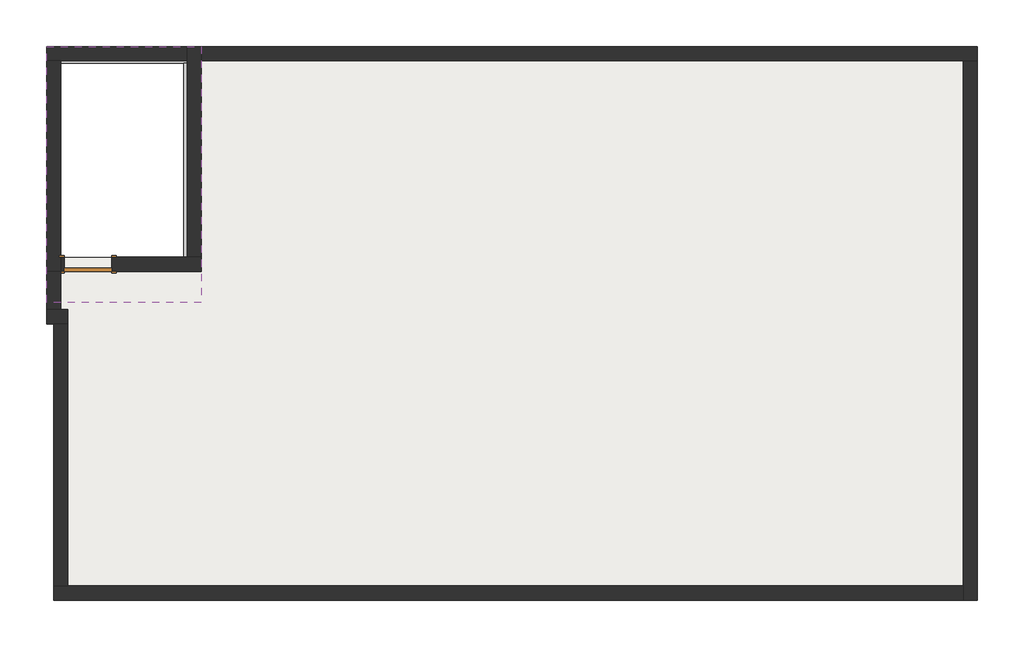
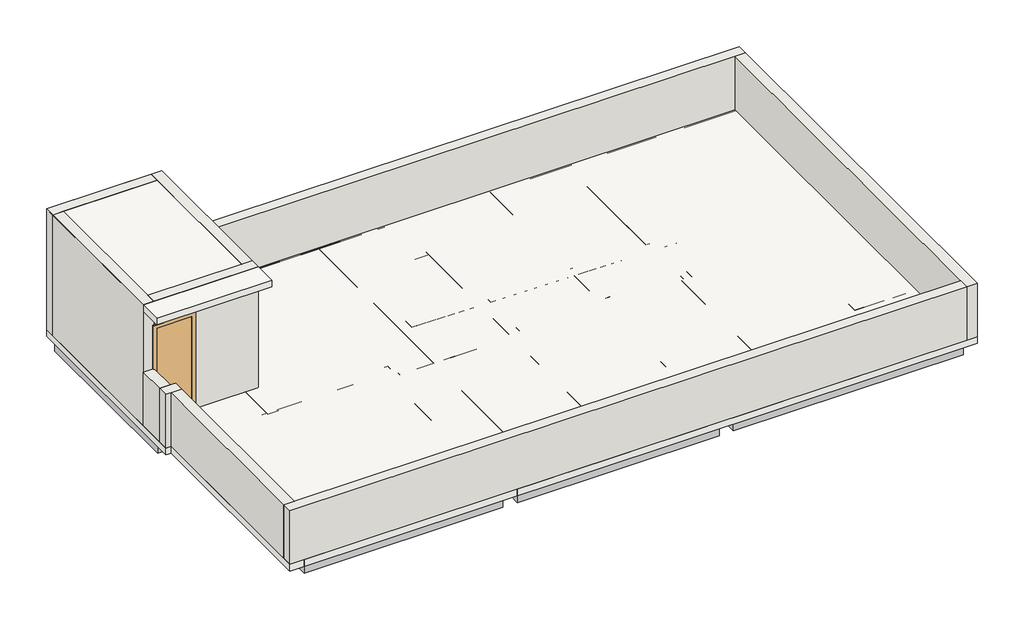
# One storey: 16 beams, 10 walls, 2 slabs, 1 door.
"""IFC4 building model written with IfcOpenShell, lengths in millimetres."""

from ifc_helpers import new_model, si_unit, frame, origin, place, context, project, spatial, polyline, outline, extrude, faceted_brep, transform, mapped, element, save
from components import door_bb98abfd

model = new_model("IFC4")

# Units and contexts
model_context = context("Model", 3, world=origin())
ifc_project = project(units=[si_unit("LENGTHUNIT", "METRE", prefix="MILLI")], contexts=[model_context])

# Site, building, storey
site = spatial("IfcSite", under=ifc_project)
building = spatial("IfcBuilding", under=site)
storey = spatial("IfcBuildingStorey", under=building, Elevation=10210.8)

# Beams
placement = place(None, origin())
element("IfcBeam", 1, ObjectType="Concrete-Rectangular Beam", at=placement, inside=storey, context=model_context, shape_type="Brep", body=[
    faceted_brep([(-12643.368339, 9510.993496, 10210.8), (-12643.368339, 9282.393496, 10210.8), (-10681.218339, 9282.393496, 10210.8), (-10452.618339, 9282.393496, 10210.8), (-7176.018339, 9282.393496, 10210.8), (-6947.418339, 9282.393496, 10210.8), (-5499.618339, 9282.393496, 10210.8), (-5271.018339, 9282.393496, 10210.8), (-3492.916739, 9282.393496, 10210.8), (-3264.316739, 9282.393496, 10210.8), (-1842.018339, 9282.393496, 10210.8), (-1613.418339, 9282.393496, 10210.8), (1790.181661, 9282.393496, 10210.8), (1790.181661, 9510.993496, 10210.8), (-1575.318339, 9510.993496, 10210.8), (-1575.318339, 9320.493496, 10210.8), (-1880.118339, 9320.493496, 10210.8), (-1880.118339, 9510.993496, 10210.8), (-6909.318339, 9510.993496, 10210.8), (-6909.318339, 9320.493496, 10210.8), (-7214.118339, 9320.493496, 10210.8), (-7214.118339, 9510.993496, 10210.8), (-10414.518339, 9510.993496, 10210.8), (-10414.518339, 9320.493496, 10210.8), (-10719.318339, 9320.493496, 10210.8), (-10719.318339, 9510.993496, 10210.8), (-12643.368339, 9282.393496, 9906.0), (-10681.218339, 9282.393496, 9906.0), (-10452.618339, 9282.393496, 9906.0), (-7176.018339, 9282.393496, 9906.0), (-6947.418339, 9282.393496, 9906.0), (-5499.618339, 9282.393496, 9906.0), (-5271.018339, 9282.393496, 9906.0), (-3492.916739, 9282.393496, 9906.0), (-3264.316739, 9282.393496, 9906.0), (-1842.018339, 9282.393496, 9906.0), (-1613.418339, 9282.393496, 9906.0), (1790.181661, 9282.393496, 9906.0), (-12643.368339, 9510.993496, 9906.0), (-10719.318339, 9510.993496, 9906.0), (-10719.318339, 9320.493496, 9906.0), (-10414.518339, 9320.493496, 9906.0), (-10414.518339, 9510.993496, 9906.0), (-7214.118339, 9510.993496, 9906.0), (-7214.118339, 9320.493496, 9906.0), (-6909.318339, 9320.493496, 9906.0), (-6909.318339, 9510.993496, 9906.0), (-1880.118339, 9510.993496, 9906.0), (-1880.118339, 9320.493496, 9906.0), (-1575.318339, 9320.493496, 9906.0), (-1575.318339, 9510.993496, 9906.0), (1790.181661, 9510.993496, 9906.0)], [[[0, 1, 2, 3, 4, 5, 6, 7, 8, 9, 10, 11, 12, 13, 14, 15, 16, 17, 18, 19, 20, 21, 22, 23, 24, 25]], [[1, 26, 27, 28, 29, 30, 31, 32, 33, 34, 35, 36, 37, 12, 11, 10, 9, 8, 7, 6, 5, 4, 3, 2]], [[26, 38, 39, 40, 41, 42, 43, 44, 45, 46, 47, 48, 49, 50, 51, 37, 36, 35, 34, 33, 32, 31, 30, 29, 28, 27]], [[13, 51, 50, 14]], [[1, 0, 38, 26]], [[13, 12, 37, 51]], [[41, 23, 22, 42]], [[23, 41, 40, 24]], [[24, 40, 39, 25]], [[38, 0, 25, 39]], [[45, 19, 18, 46]], [[19, 45, 44, 20]], [[20, 44, 43, 21]], [[42, 22, 21, 43]], [[49, 15, 14, 50]], [[15, 49, 48, 16]], [[16, 48, 47, 17]], [[46, 18, 17, 47]]]),
])
element("IfcBeam", 2, ObjectType="Concrete-Rectangular Beam", at=placement, inside=storey, context=model_context, shape_type="Brep", body=[
    faceted_brep([(1790.181661, 913.093496, 10210.8), (2018.781661, 913.093496, 10210.8), (2018.781661, 4958.043496, 10210.8), (1790.181661, 4958.043496, 10210.8), (1790.181661, 2792.693496, 10210.8), (1790.181661, 2564.093496, 10210.8), (1790.181661, 913.093496, 9906.0), (1790.181661, 4958.043496, 9906.0), (1790.181661, 2792.693496, 9906.0), (1790.181661, 2564.093496, 9906.0), (2018.781661, 913.093496, 9906.0), (2018.781661, 4958.043496, 9906.0)], [[[0, 1, 2, 3, 4, 5]], [[6, 0, 5, 4, 3, 7, 8, 9]], [[10, 6, 9, 8, 7, 11]], [[1, 10, 11, 2]], [[1, 0, 6, 10]], [[3, 2, 11, 7]]]),
    faceted_brep([(1790.181661, 9244.293496, 10210.8), (2018.781661, 9244.293496, 10210.8), (2018.781661, 9244.293496, 9906.0), (1790.181661, 9244.293496, 9906.0), (2018.781661, 5262.843496, 10210.8), (1790.181661, 5262.843496, 10210.8), (1790.181661, 5262.843496, 9906.0), (2018.781661, 5262.843496, 9906.0)], [[[0, 1, 2, 3]], [[4, 5, 6, 7]], [[1, 0, 5, 4]], [[0, 3, 6, 5]], [[3, 2, 7, 6]], [[2, 1, 4, 7]]]),
])
element("IfcBeam", 3, ObjectType="Concrete-Rectangular Beam", at=placement, inside=storey, context=model_context, shape_type="Brep", body=[
    faceted_brep([(-12452.868339, 913.093496, 10210.8), (-12452.868339, 684.493496, 10210.8), (-8179.318339, 684.493496, 10210.8), (-8179.318339, 913.093496, 10210.8), (-12452.868339, 913.093496, 9906.0), (-8179.318339, 913.093496, 9906.0), (-12452.868339, 684.493496, 9906.0), (-8179.318339, 684.493496, 9906.0)], [[[0, 1, 2, 3]], [[4, 0, 3, 5]], [[6, 4, 5, 7]], [[1, 6, 7, 2]], [[1, 0, 4, 6]], [[3, 2, 7, 5]]]),
    faceted_brep([(1713.981661, 913.093496, 10210.8), (1713.981661, 684.493496, 10210.8), (1713.981661, 684.493496, 9906.0), (1713.981661, 913.093496, 9906.0), (-3226.216739, 684.493496, 10210.8), (-3226.216739, 913.093496, 10210.8), (-3226.216739, 913.093496, 9906.0), (-3226.216739, 684.493496, 9906.0), (469.381661, 913.093496, 10210.8), (240.781661, 913.093496, 10210.8), (-1613.418339, 913.093496, 10210.8), (-1842.018339, 913.093496, 10210.8), (469.381661, 913.093496, 9906.0), (240.781661, 913.093496, 9906.0), (-1613.418339, 913.093496, 9906.0), (-1842.018339, 913.093496, 9906.0)], [[[0, 1, 2, 3]], [[4, 5, 6, 7]], [[1, 0, 8, 9, 10, 11, 5, 4]], [[0, 3, 12, 13, 14, 15, 6, 5, 11, 10, 9, 8]], [[3, 2, 7, 6, 15, 14, 13, 12]], [[2, 1, 4, 7]]]),
    faceted_brep([(-7874.518339, 684.493496, 10210.8), (-7874.518339, 913.093496, 10210.8), (-7874.518339, 913.093496, 9906.0), (-7874.518339, 684.493496, 9906.0), (-3531.016739, 684.493496, 10210.8), (-3531.016739, 913.093496, 10210.8), (-5271.018339, 913.093496, 10210.8), (-5499.618339, 913.093496, 10210.8), (-6947.418339, 913.093496, 10210.8), (-7176.018339, 913.093496, 10210.8), (-3531.016739, 913.093496, 9906.0), (-5271.018339, 913.093496, 9906.0), (-5499.618339, 913.093496, 9906.0), (-6947.418339, 913.093496, 9906.0), (-7176.018339, 913.093496, 9906.0), (-3531.016739, 684.493496, 9906.0)], [[[0, 1, 2, 3]], [[1, 0, 4, 5, 6, 7, 8, 9]], [[2, 1, 9, 8, 7, 6, 5, 10, 11, 12, 13, 14]], [[3, 2, 14, 13, 12, 11, 10, 15]], [[0, 3, 15, 4]], [[5, 4, 15, 10]]]),
])
element("IfcBeam", 4, ObjectType="Concrete-Rectangular Beam", at=placement, inside=storey, context=model_context, shape_type="SweptSolid", body=[
    extrude(outline(polyline([(-12871.968339, 9244.293496), (-12643.368339, 9244.293496), (-12643.368339, 5415.243496), (-12871.968339, 5415.243496), (-12871.968339, 9244.293496)])), frame((0.0, 0.0, 9906.0), z_axis=(0.0, 0.0, 1.0), x_axis=(1.0, 0.0, 0.0)), (0.0, 0.0, 1.0), 304.8),
])
element("IfcBeam", 5, ObjectType="Concrete-Rectangular Beam", at=placement, inside=storey, context=model_context, shape_type="Brep", body=[
    faceted_brep([(-10452.618339, 5110.443496, 10210.8), (-10681.218339, 5110.443496, 10210.8), (-10681.218339, 5110.443496, 9906.0), (-10452.618339, 5110.443496, 9906.0), (-10452.618339, 5148.543496, 10210.8), (-10452.618339, 5377.143496, 10210.8), (-10452.618339, 9282.393496, 10210.8), (-10681.218339, 9282.393496, 10210.8), (-10681.218339, 5377.143496, 10210.8), (-10681.218339, 5148.543496, 10210.8), (-10681.218339, 9282.393496, 9906.0), (-10681.218339, 5377.143496, 9906.0), (-10681.218339, 5148.543496, 9906.0), (-10452.618339, 9282.393496, 9906.0), (-10452.618339, 5377.143496, 9906.0), (-10452.618339, 5148.543496, 9906.0)], [[[0, 1, 2, 3]], [[1, 0, 4, 5, 6, 7, 8, 9]], [[2, 1, 9, 8, 7, 10, 11, 12]], [[3, 2, 12, 11, 10, 13, 14, 15]], [[0, 3, 15, 14, 13, 6, 5, 4]], [[7, 6, 13, 10]]]),
])
element("IfcBeam", 6, ObjectType="Concrete-Rectangular Beam", at=placement, inside=storey, context=model_context, shape_type="Brep", body=[
    faceted_brep([(-10452.618339, 5377.143496, 10210.8), (-10452.618339, 5148.543496, 10210.8), (-8274.568339, 5148.543496, 10210.8), (-8274.568339, 5339.043496, 10210.8), (-7969.768339, 5339.043496, 10210.8), (-7969.768339, 5148.543496, 10210.8), (-7912.618339, 5148.543496, 10210.8), (-7912.618339, 5224.743496, 10210.8), (-7912.618339, 5377.143496, 10210.8), (-7912.618339, 5148.543496, 9906.0), (-7969.768339, 5148.543496, 9906.0), (-10452.618339, 5148.543496, 9906.0), (-10452.618339, 5377.143496, 9906.0), (-7912.618339, 5377.143496, 9906.0), (-7912.618339, 5224.743496, 9906.0), (-7969.768339, 5339.043496, 9906.0), (-8274.568339, 5339.043496, 9906.0), (-8274.568339, 5148.543496, 9906.0)], [[[0, 1, 2, 3, 4, 5, 6, 7, 8]], [[9, 6, 5, 10]], [[11, 12, 13, 14, 9, 10, 15, 16, 17]], [[12, 0, 8, 13]], [[1, 0, 12, 11]], [[8, 7, 6, 9, 14, 13]], [[16, 3, 2, 17]], [[3, 16, 15, 4]], [[4, 15, 10, 5]], [[1, 11, 17, 2]]]),
    faceted_brep([(-12643.368339, 5148.543496, 10210.8), (-12643.368339, 5377.143496, 10210.8), (-12643.368339, 5377.143496, 9906.0), (-12643.368339, 5148.543496, 9906.0), (-10681.218339, 5377.143496, 10210.8), (-10681.218339, 5148.543496, 10210.8), (-10681.218339, 5148.543496, 9906.0), (-10681.218339, 5377.143496, 9906.0)], [[[0, 1, 2, 3]], [[4, 5, 6, 7]], [[1, 0, 5, 4]], [[3, 2, 7, 6]], [[2, 1, 4, 7]], [[0, 3, 6, 5]]]),
])
element("IfcBeam", 7, ObjectType="Concrete-Rectangular Beam", at=placement, inside=storey, context=model_context, shape_type="Brep", body=[
    faceted_brep([(-8141.218339, 913.093496, 10210.8), (-7912.618339, 913.093496, 10210.8), (-7912.618339, 4996.143496, 10210.8), (-7912.618339, 5148.543496, 10210.8), (-7969.768339, 5148.543496, 10210.8), (-7969.768339, 5110.443496, 10210.8), (-8141.218339, 5110.443496, 10210.8), (-7912.618339, 913.093496, 9906.0), (-7912.618339, 4996.143496, 9906.0), (-7912.618339, 5148.543496, 9906.0), (-8141.218339, 913.093496, 9906.0), (-8141.218339, 5110.443496, 9906.0), (-7969.768339, 5110.443496, 9906.0), (-7969.768339, 5148.543496, 9906.0)], [[[0, 1, 2, 3, 4, 5, 6]], [[1, 7, 8, 9, 3, 2]], [[7, 10, 11, 12, 13, 9, 8]], [[10, 0, 6, 11]], [[3, 9, 13, 4]], [[1, 0, 10, 7]], [[5, 12, 11, 6]], [[12, 5, 4, 13]]]),
])
element("IfcBeam", 8, ObjectType="Concrete-Rectangular Beam", at=placement, inside=storey, context=model_context, shape_type="Brep", body=[
    faceted_brep([(-6947.418339, 9282.393496, 10210.8), (-7176.018339, 9282.393496, 10210.8), (-7176.018339, 5224.743496, 10210.8), (-7176.018339, 4996.143496, 10210.8), (-7176.018339, 913.093496, 10210.8), (-6947.418339, 913.093496, 10210.8), (-6947.418339, 4996.143496, 10210.8), (-6947.418339, 5224.743496, 10210.8), (-6947.418339, 6213.330971, 10210.8), (-6947.418339, 6441.9657932, 10210.8), (-6947.418339, 8094.943496, 10210.8), (-6947.418339, 8323.543496, 10210.8), (-7176.018339, 9282.393496, 9906.0), (-7176.018339, 5224.743496, 9906.0), (-7176.018339, 4996.143496, 9906.0), (-7176.018339, 913.093496, 9906.0), (-6947.418339, 9282.393496, 9906.0), (-6947.418339, 8323.543496, 9906.0), (-6947.418339, 8094.943496, 9906.0), (-6947.418339, 6441.9657932, 9906.0), (-6947.418339, 6213.330971, 9906.0), (-6947.418339, 5224.743496, 9906.0), (-6947.418339, 4996.143496, 9906.0), (-6947.418339, 913.093496, 9906.0)], [[[0, 1, 2, 3, 4, 5, 6, 7, 8, 9, 10, 11]], [[1, 12, 13, 14, 15, 4, 3, 2]], [[12, 16, 17, 18, 19, 20, 21, 22, 23, 15, 14, 13]], [[16, 0, 11, 10, 9, 8, 7, 6, 5, 23, 22, 21, 20, 19, 18, 17]], [[1, 0, 16, 12]], [[5, 4, 15, 23]]]),
])
element("IfcBeam", 9, ObjectType="Concrete-Rectangular Beam", at=placement, inside=storey, context=model_context, shape_type="Brep", body=[
    faceted_brep([(-5271.018339, 9282.393496, 10210.8), (-5499.618339, 9282.393496, 10210.8), (-5499.618339, 8323.543496, 10210.8), (-5499.618339, 8094.943496, 10210.8), (-5499.618339, 6416.6943502, 10210.8), (-5499.618339, 6188.059528, 10210.8), (-5499.618339, 5224.743496, 10210.8), (-5499.618339, 4996.143496, 10210.8), (-5499.618339, 913.093496, 10210.8), (-5271.018339, 913.093496, 10210.8), (-5271.018339, 4996.143496, 10210.8), (-5271.018339, 5224.743496, 10210.8), (-5271.018339, 6184.0693001, 10210.8), (-5271.018339, 6412.7041223, 10210.8), (-5499.618339, 9282.393496, 9906.0), (-5499.618339, 8323.543496, 9906.0), (-5499.618339, 8094.943496, 9906.0), (-5499.618339, 6416.6943502, 9906.0), (-5499.618339, 6188.059528, 9906.0), (-5499.618339, 5224.743496, 9906.0), (-5499.618339, 4996.143496, 9906.0), (-5499.618339, 913.093496, 9906.0), (-5271.018339, 9282.393496, 9906.0), (-5271.018339, 6412.7041223, 9906.0), (-5271.018339, 6184.0693001, 9906.0), (-5271.018339, 5224.743496, 9906.0), (-5271.018339, 4996.143496, 9906.0), (-5271.018339, 913.093496, 9906.0)], [[[0, 1, 2, 3, 4, 5, 6, 7, 8, 9, 10, 11, 12, 13]], [[1, 14, 15, 16, 17, 18, 19, 20, 21, 8, 7, 6, 5, 4, 3, 2]], [[14, 22, 23, 24, 25, 26, 27, 21, 20, 19, 18, 17, 16, 15]], [[22, 0, 13, 12, 11, 10, 9, 27, 26, 25, 24, 23]], [[1, 0, 22, 14]], [[9, 8, 21, 27]]]),
])
element("IfcBeam", 10, ObjectType="Concrete-Rectangular Beam", at=placement, inside=storey, context=model_context, shape_type="SweptSolid", body=[
    extrude(outline(polyline([(-6947.418339, 8094.943496), (-6947.418339, 8323.543496), (-5499.618339, 8323.543496), (-5499.618339, 8094.943496), (-6947.418339, 8094.943496)])), frame((0.0, 0.0, 9906.0), z_axis=(0.0, 0.0, 1.0), x_axis=(1.0, 0.0, 0.0)), (0.0, 0.0, 1.0), 304.8),
])
element("IfcBeam", 11, ObjectType="Concrete-Rectangular Beam", at=placement, inside=storey, context=model_context, shape_type="Brep", body=[
    faceted_brep([(1778.1302181, 6289.6607766, 10210.8), (1774.140598, 6061.0955935, 10210.8), (1774.140598, 6061.0955935, 9906.0), (1778.1302181, 6289.6607766, 9906.0), (-1613.418339, 6348.8604768, 10210.8), (-1842.018339, 6352.8507047, 10210.8), (-3264.316739, 6377.6770156, 10210.8), (-3492.916739, 6381.6672435, 10210.8), (-5271.018339, 6412.7041223, 10210.8), (-5271.018339, 6184.0693001, 10210.8), (-3492.916739, 6153.0324213, 10210.8), (-3264.316739, 6149.0421934, 10210.8), (-1842.018339, 6124.2158825, 10210.8), (-1613.418339, 6120.2256547, 10210.8), (-5271.018339, 6184.0693001, 9906.0), (-3492.916739, 6153.0324213, 9906.0), (-3264.316739, 6149.0421934, 9906.0), (-1842.018339, 6124.2158825, 9906.0), (-1613.418339, 6120.2256547, 9906.0), (-5271.018339, 6412.7041223, 9906.0), (-3492.916739, 6381.6672435, 9906.0), (-3264.316739, 6377.6770156, 9906.0), (-1842.018339, 6352.8507047, 9906.0), (-1613.418339, 6348.8604768, 9906.0)], [[[0, 1, 2, 3]], [[1, 0, 4, 5, 6, 7, 8, 9, 10, 11, 12, 13]], [[2, 1, 13, 12, 11, 10, 9, 14, 15, 16, 17, 18]], [[3, 2, 18, 17, 16, 15, 14, 19, 20, 21, 22, 23]], [[0, 3, 23, 22, 21, 20, 19, 8, 7, 6, 5, 4]], [[9, 8, 19, 14]]]),
    faceted_brep([(-6947.418339, 6213.330971, 10210.8), (-6947.418339, 6441.9657932, 10210.8), (-6947.418339, 6441.9657932, 9906.0), (-6947.418339, 6213.330971, 9906.0), (-5499.618339, 6416.6943502, 10210.8), (-5499.618339, 6188.059528, 10210.8), (-5499.618339, 6188.059528, 9906.0), (-5499.618339, 6416.6943502, 9906.0)], [[[0, 1, 2, 3]], [[4, 5, 6, 7]], [[1, 0, 5, 4]], [[0, 3, 6, 5]], [[3, 2, 7, 6]], [[2, 1, 4, 7]]]),
])
element("IfcBeam", 12, ObjectType="Concrete-Rectangular Beam", at=placement, inside=storey, context=model_context, shape_type="Brep", body=[
    faceted_brep([(-1842.018339, 913.093496, 10210.8), (-1613.418339, 913.093496, 10210.8), (-1613.418339, 4996.143496, 10210.8), (-1613.418339, 5224.743496, 10210.8), (-1613.418339, 6120.2256547, 10210.8), (-1842.018339, 6124.2158825, 10210.8), (-1842.018339, 5281.893496, 10210.8), (-1784.868339, 5281.893496, 10210.8), (-1784.868339, 5053.293496, 10210.8), (-1842.018339, 5053.293496, 10210.8), (-1842.018339, 4996.143496, 10210.8), (-1842.018339, 913.093496, 9906.0), (-1842.018339, 5053.293496, 9906.0), (-1842.018339, 4996.143496, 9906.0), (-1613.418339, 913.093496, 9906.0), (-1784.868339, 5053.293496, 9906.0), (-1784.868339, 5281.893496, 9906.0), (-1842.018339, 5281.893496, 9906.0), (-1842.018339, 6124.2158825, 9906.0), (-1613.418339, 6120.2256547, 9906.0), (-1613.418339, 5224.743496, 9906.0), (-1613.418339, 4996.143496, 9906.0)], [[[0, 1, 2, 3, 4, 5, 6, 7, 8, 9, 10]], [[11, 0, 10, 9, 12, 13]], [[14, 11, 13, 12, 15, 16, 17, 18, 19, 20, 21]], [[1, 14, 21, 20, 19, 4, 3, 2]], [[1, 0, 11, 14]], [[5, 4, 19, 18]], [[8, 15, 12, 9]], [[16, 7, 6, 17]], [[7, 16, 15, 8]], [[5, 18, 17, 6]]]),
    faceted_brep([(-1842.018339, 9282.393496, 10210.8), (-1613.418339, 9282.393496, 10210.8), (-1613.418339, 9282.393496, 9906.0), (-1842.018339, 9282.393496, 9906.0), (-1613.418339, 6348.8604768, 10210.8), (-1842.018339, 6352.8507047, 10210.8), (-1842.018339, 6352.8507047, 9906.0), (-1613.418339, 6348.8604768, 9906.0)], [[[0, 1, 2, 3]], [[4, 5, 6, 7]], [[1, 0, 5, 4]], [[3, 2, 7, 6]], [[2, 1, 4, 7]], [[0, 3, 6, 5]]]),
])
element("IfcBeam", 13, ObjectType="Concrete-Rectangular Beam", at=placement, inside=storey, context=model_context, shape_type="Brep", body=[
    faceted_brep([(-7176.018339, 4996.143496, 10210.8), (-7176.018339, 5224.743496, 10210.8), (-7912.618339, 5224.743496, 10210.8), (-7912.618339, 5148.543496, 10210.8), (-7912.618339, 4996.143496, 10210.8), (-7176.018339, 5224.743496, 9906.0), (-7912.618339, 5224.743496, 9906.0), (-7176.018339, 4996.143496, 9906.0), (-7912.618339, 4996.143496, 9906.0), (-7912.618339, 5148.543496, 9906.0)], [[[0, 1, 2, 3, 4]], [[1, 5, 6, 2]], [[5, 7, 8, 9, 6]], [[4, 8, 7, 0]], [[1, 0, 7, 5]], [[8, 4, 3, 2, 6, 9]]]),
    faceted_brep([(-6947.418339, 4996.143496, 10210.8), (-6947.418339, 5224.743496, 10210.8), (-6947.418339, 5224.743496, 9906.0), (-6947.418339, 4996.143496, 9906.0), (-5499.618339, 4996.143496, 10210.8), (-5499.618339, 5224.743496, 10210.8), (-5499.618339, 5224.743496, 9906.0), (-5499.618339, 4996.143496, 9906.0)], [[[0, 1, 2, 3]], [[1, 0, 4, 5]], [[2, 1, 5, 6]], [[3, 2, 6, 7]], [[0, 3, 7, 4]], [[5, 4, 7, 6]]]),
    faceted_brep([(-5271.018339, 4996.143496, 10210.8), (-5271.018339, 5224.743496, 10210.8), (-5271.018339, 5224.743496, 9906.0), (-5271.018339, 4996.143496, 9906.0), (-3492.916739, 4996.143496, 10210.8), (-3264.316739, 4996.143496, 10210.8), (-1842.018339, 4996.143496, 10210.8), (-1842.018339, 5053.293496, 10210.8), (-2089.668339, 5053.293496, 10210.8), (-2089.668339, 5224.743496, 10210.8), (-3264.316739, 5224.743496, 10210.8), (-3492.916739, 5224.743496, 10210.8), (-2089.668339, 5224.743496, 9906.0), (-3264.316739, 5224.743496, 9906.0), (-3492.916739, 5224.743496, 9906.0), (-2089.668339, 5053.293496, 9906.0), (-1842.018339, 5053.293496, 9906.0), (-1842.018339, 4996.143496, 9906.0), (-3264.316739, 4996.143496, 9906.0), (-3492.916739, 4996.143496, 9906.0)], [[[0, 1, 2, 3]], [[1, 0, 4, 5, 6, 7, 8, 9, 10, 11]], [[2, 1, 11, 10, 9, 12, 13, 14]], [[3, 2, 14, 13, 12, 15, 16, 17, 18, 19]], [[0, 3, 19, 18, 17, 6, 5, 4]], [[6, 17, 16, 7]], [[15, 8, 7, 16]], [[8, 15, 12, 9]]]),
    faceted_brep([(-1613.418339, 4996.143496, 10210.8), (-1613.418339, 5224.743496, 10210.8), (-1613.418339, 5224.743496, 9906.0), (-1613.418339, 4996.143496, 9906.0), (240.781661, 4996.143496, 10210.8), (469.381661, 4996.143496, 10210.8), (1790.181661, 4996.143496, 10210.8), (1790.181661, 5224.743496, 10210.8), (1790.181661, 5224.743496, 9906.0), (1790.181661, 4996.143496, 9906.0), (469.381661, 4996.143496, 9906.0), (240.781661, 4996.143496, 9906.0)], [[[0, 1, 2, 3]], [[1, 0, 4, 5, 6, 7]], [[3, 2, 8, 9, 10, 11]], [[0, 3, 11, 10, 9, 6, 5, 4]], [[2, 1, 7, 8]], [[7, 6, 9, 8]]]),
])
element("IfcBeam", 14, ObjectType="Concrete-Rectangular Beam", at=placement, inside=storey, context=model_context, shape_type="SweptSolid", body=[
    extrude(outline(polyline([(-3492.916739, 9282.393496), (-3264.316739, 9282.393496), (-3264.316739, 6377.6770156), (-3492.916739, 6381.6672435), (-3492.916739, 9282.393496)])), frame((0.0, 0.0, 9906.0), z_axis=(0.0, 0.0, 1.0), x_axis=(1.0, 0.0, 0.0)), (0.0, 0.0, 1.0), 304.8),
    extrude(outline(polyline([(-3492.916739, 6153.0324213), (-3264.316739, 6149.0421934), (-3264.316739, 5224.743496), (-3492.916739, 5224.743496), (-3492.916739, 6153.0324213)])), frame((0.0, 0.0, 9906.0), z_axis=(0.0, 0.0, 1.0), x_axis=(1.0, 0.0, 0.0)), (0.0, 0.0, 1.0), 304.8),
    extrude(outline(polyline([(-3492.916739, 4996.143496), (-3264.316739, 4996.143496), (-3264.316739, 913.093496), (-3492.916739, 913.093496), (-3492.916739, 4996.143496)])), frame((0.0, 0.0, 9906.0), z_axis=(0.0, 0.0, 1.0), x_axis=(1.0, 0.0, 0.0)), (0.0, 0.0, 1.0), 304.8),
])
element("IfcBeam", 15, ObjectType="Concrete-Rectangular Beam", at=placement, inside=storey, context=model_context, shape_type="Brep", body=[
    faceted_brep([(240.781661, 913.093496, 10210.8), (469.381661, 913.093496, 10210.8), (469.381661, 2564.093496, 10210.8), (469.381661, 2792.693496, 10210.8), (469.381661, 4996.143496, 10210.8), (240.781661, 4996.143496, 10210.8), (469.381661, 913.093496, 9906.0), (469.381661, 2564.093496, 9906.0), (469.381661, 2792.693496, 9906.0), (469.381661, 4996.143496, 9906.0), (240.781661, 913.093496, 9906.0), (240.781661, 4996.143496, 9906.0)], [[[0, 1, 2, 3, 4, 5]], [[1, 6, 7, 8, 9, 4, 3, 2]], [[6, 10, 11, 9, 8, 7]], [[10, 0, 5, 11]], [[1, 0, 10, 6]], [[5, 4, 9, 11]]]),
])
element("IfcBeam", 16, ObjectType="Concrete-Rectangular Beam", at=placement, inside=storey, context=model_context, shape_type="SweptSolid", body=[
    extrude(outline(polyline([(1790.181661, 2792.693496), (1790.181661, 2564.093496), (469.381661, 2564.093496), (469.381661, 2792.693496), (1790.181661, 2792.693496)])), frame((0.0, 0.0, 9906.0), z_axis=(0.0, 0.0, 1.0), x_axis=(1.0, 0.0, 0.0)), (0.0, 0.0, 1.0), 304.8),
])

# Door
door_shape = door_bb98abfd(model_context)
element("IfcDoor", 17, ObjectType="Single-Flush : 30\" x 84\"", at=placement, inside=storey, context=model_context, shape_type="MappedRepresentation", body=[
    mapped(door_shape, transform((-12211.568339, 6062.943496, 10210.8), x_axis=(-1.0, 0.0, 0.0), y_axis=(0.0, -1.0, 0.0), z_axis=(0.0, 0.0, 1.0))),
])

# Slabs
element("IfcSlab", 18, ObjectType="Generic - 6\"", at=placement, inside=storey, context=model_context, shape_type="SweptSolid", body=[
    extrude(outline(polyline([(2018.781661, 9549.093496), (2018.781661, 684.493496), (-12757.668339, 684.493496), (-12757.668339, 5110.443496), (-12871.968339, 5110.443496), (-12871.968339, 9549.093496), (2018.781661, 9549.093496)]), holes=[polyline([(-10624.068339, 9320.493496), (-12643.368339, 9320.493496), (-12643.368339, 6177.243496), (-10624.068339, 6177.243496), (-10624.068339, 9320.493496)])]), frame((0.0, 0.0, 10058.4), z_axis=(0.0, 0.0, 1.0), x_axis=(1.0, 0.0, 0.0)), (0.0, 0.0, 1.0), 152.4),
])
element("IfcSlab", 19, ObjectType="Generic - 6\"", at=placement, inside=storey, context=model_context, shape_type="SweptSolid", body=[
    extrude(outline(polyline([(-10395.468339, 9549.093496), (-10395.468339, 5453.343496), (-12871.968339, 5453.343496), (-12871.968339, 9549.093496), (-10395.468339, 9549.093496)])), frame((0.0, 0.0, 12801.6), z_axis=(0.0, 0.0, 1.0), x_axis=(1.0, 0.0, 0.0)), (0.0, 0.0, 1.0), 152.4),
])

# Walls
element("IfcWall", 20, ObjectType="Generic - 9\"", at=placement, inside=storey, context=model_context, shape_type="Brep", body=[
    faceted_brep([(-12871.968339, 9320.493496, 10210.8), (-12871.968339, 5948.643496, 10210.8), (-12871.968339, 5948.643496, 11430.0), (-12871.968339, 5948.643496, 12954.0), (-12871.968339, 9320.493496, 12954.0), (-12643.368339, 9320.493496, 10210.8), (-12643.368339, 9320.493496, 12954.0), (-12643.368339, 6177.243496, 12954.0), (-12643.368339, 5948.643496, 12954.0), (-12643.368339, 5948.643496, 11430.0), (-12643.368339, 5948.643496, 10210.8), (-12643.368339, 6177.243496, 10210.8)], [[[0, 1, 2, 3, 4]], [[5, 6, 7, 8, 9, 10, 11]], [[1, 0, 5, 11, 10]], [[4, 3, 8, 7, 6]], [[0, 4, 6, 5]], [[1, 10, 9, 8, 3, 2]]]),
])
element("IfcWall", 21, ObjectType="Generic - 9\"", at=placement, inside=storey, context=model_context, shape_type="Brep", body=[
    faceted_brep([(-12643.368339, 5948.643496, 10210.8), (-12592.568339, 5948.643496, 10210.8), (-12592.568339, 5948.643496, 12344.4), (-11830.568339, 5948.643496, 12344.4), (-11830.568339, 5948.643496, 10210.8), (-10395.468339, 5948.643496, 10210.8), (-10395.468339, 5948.643496, 12954.0), (-12643.368339, 5948.643496, 12954.0), (-12592.568339, 6177.243496, 12344.4), (-12592.568339, 6177.243496, 10210.8), (-12643.368339, 6177.243496, 10210.8), (-12643.368339, 6177.243496, 12954.0), (-10624.068339, 6177.243496, 12954.0), (-10395.468339, 6177.243496, 12954.0), (-10395.468339, 6177.243496, 10210.8), (-10624.068339, 6177.243496, 10210.8), (-11830.568339, 6177.243496, 10210.8), (-11830.568339, 6177.243496, 12344.4)], [[[0, 1, 2, 3, 4, 5, 6, 7]], [[8, 9, 10, 11, 12, 13, 14, 15, 16, 17]], [[10, 9, 1, 0]], [[16, 15, 14, 5, 4]], [[7, 6, 13, 12, 11]], [[6, 5, 14, 13]], [[2, 1, 9, 8]], [[3, 2, 8, 17]], [[4, 3, 17, 16]], [[7, 11, 10, 0]]]),
])
element("IfcWall", 22, ObjectType="Generic - 9\"", at=placement, inside=storey, context=model_context, shape_type="Brep", body=[
    faceted_brep([(-10395.468339, 6177.243496, 10210.8), (-10395.468339, 9320.493496, 10210.8), (-10395.468339, 9549.093496, 10210.8), (-10395.468339, 9549.093496, 11430.0), (-10395.468339, 9549.093496, 12954.0), (-10395.468339, 6177.243496, 12954.0), (-10624.068339, 6177.243496, 10210.8), (-10624.068339, 6177.243496, 12954.0), (-10624.068339, 9320.493496, 12954.0), (-10624.068339, 9549.093496, 12954.0), (-10624.068339, 9549.093496, 10210.8), (-10624.068339, 9320.493496, 10210.8)], [[[0, 1, 2, 3, 4, 5]], [[6, 7, 8, 9, 10, 11]], [[2, 1, 0, 6, 11, 10]], [[5, 4, 9, 8, 7]], [[0, 5, 7, 6]], [[2, 10, 9, 4, 3]]]),
])
element("IfcWall", 23, ObjectType="Generic - 9\"", at=placement, inside=storey, context=model_context, shape_type="Brep", body=[
    faceted_brep([(-10624.068339, 9549.093496, 12954.0), (-10624.068339, 9549.093496, 10210.8), (-12871.968339, 9549.093496, 10210.8), (-12871.968339, 9549.093496, 12954.0), (-10624.068339, 9320.493496, 10210.8), (-10624.068339, 9320.493496, 12954.0), (-12643.368339, 9320.493496, 12954.0), (-12871.968339, 9320.493496, 12954.0), (-12871.968339, 9320.493496, 10210.8), (-12643.368339, 9320.493496, 10210.8)], [[[0, 1, 2, 3]], [[4, 5, 6, 7, 8, 9]], [[2, 1, 4, 9, 8]], [[0, 3, 7, 6, 5]], [[3, 2, 8, 7]], [[0, 5, 4, 1]]]),
])
element("IfcWall", 24, ObjectType="Generic - 9\"", at=placement, inside=storey, context=model_context, shape_type="Brep", body=[
    faceted_brep([(-10395.468339, 9320.493496, 10210.8), (1790.181661, 9320.493496, 10210.8), (2018.781661, 9320.493496, 10210.8), (2018.781661, 9320.493496, 11430.0), (1790.181661, 9320.493496, 11430.0), (-10395.468339, 9320.493496, 11430.0), (-10395.468339, 9549.093496, 10210.8), (-10395.468339, 9549.093496, 11430.0), (2018.781661, 9549.093496, 11430.0), (2018.781661, 9549.093496, 10210.8)], [[[0, 1, 2, 3, 4, 5]], [[6, 7, 8, 9]], [[2, 1, 0, 6, 9]], [[5, 4, 3, 8, 7]], [[0, 5, 7, 6]], [[3, 2, 9, 8]]]),
])
element("IfcWall", 25, ObjectType="Generic - 9\"", at=placement, inside=storey, context=model_context, shape_type="Brep", body=[
    faceted_brep([(1790.181661, 9320.493496, 10210.8), (1790.181661, 913.093496, 10210.8), (1790.181661, 684.493496, 10210.8), (1790.181661, 684.493496, 11430.0), (1790.181661, 913.093496, 11430.0), (1790.181661, 9320.493496, 11430.0), (2018.781661, 9320.493496, 10210.8), (2018.781661, 9320.493496, 11430.0), (2018.781661, 684.493496, 11430.0), (2018.781661, 684.493496, 10210.8)], [[[0, 1, 2, 3, 4, 5]], [[6, 7, 8, 9]], [[2, 1, 0, 6, 9]], [[5, 4, 3, 8, 7]], [[0, 5, 7, 6]], [[3, 2, 9, 8]]]),
])
element("IfcWall", 26, ObjectType="Generic - 9\"", at=placement, inside=storey, context=model_context, shape_type="Brep", body=[
    faceted_brep([(1790.181661, 913.093496, 10210.8), (-12529.068339, 913.093496, 10210.8), (-12757.668339, 913.093496, 10210.8), (-12757.668339, 913.093496, 11430.0), (-12529.068339, 913.093496, 11430.0), (1790.181661, 913.093496, 11430.0), (1790.181661, 684.493496, 10210.8), (1790.181661, 684.493496, 11430.0), (-12757.668339, 684.493496, 11430.0), (-12757.668339, 684.493496, 10210.8)], [[[0, 1, 2, 3, 4, 5]], [[6, 7, 8, 9]], [[2, 1, 0, 6, 9]], [[5, 4, 3, 8, 7]], [[0, 5, 7, 6]], [[3, 2, 9, 8]]]),
])
element("IfcWall", 27, ObjectType="Generic - 9\"", at=placement, inside=storey, context=model_context, shape_type="SweptSolid", body=[
    extrude(outline(polyline([(-12529.068339, 5110.443496), (-12529.068339, 913.093496), (-12757.668339, 913.093496), (-12757.668339, 5110.443496), (-12529.068339, 5110.443496)])), frame((0.0, 0.0, 10210.8), z_axis=(0.0, 0.0, 1.0), x_axis=(1.0, 0.0, 0.0)), (0.0, 0.0, 1.0), 1219.2),
])
element("IfcWall", 28, ObjectType="Generic - 9\"", at=placement, inside=storey, context=model_context, shape_type="Brep", body=[
    faceted_brep([(-12529.068339, 5339.043496, 10210.8), (-12643.368339, 5339.043496, 10210.8), (-12871.968339, 5339.043496, 10210.8), (-12871.968339, 5339.043496, 11430.0), (-12643.368339, 5339.043496, 11430.0), (-12529.068339, 5339.043496, 11430.0), (-12529.068339, 5110.443496, 10210.8), (-12529.068339, 5110.443496, 11430.0), (-12757.668339, 5110.443496, 11430.0), (-12871.968339, 5110.443496, 11430.0), (-12871.968339, 5110.443496, 10210.8), (-12757.668339, 5110.443496, 10210.8)], [[[0, 1, 2, 3, 4, 5]], [[6, 7, 8, 9, 10, 11]], [[2, 1, 0, 6, 11, 10]], [[5, 4, 3, 9, 8, 7]], [[0, 5, 7, 6]], [[3, 2, 10, 9]]]),
])
element("IfcWall", 29, ObjectType="Generic - 9\"", at=placement, inside=storey, context=model_context, shape_type="SweptSolid", body=[
    extrude(outline(polyline([(-12643.368339, 5948.643496), (-12643.368339, 5339.043496), (-12871.968339, 5339.043496), (-12871.968339, 5948.643496), (-12643.368339, 5948.643496)])), frame((0.0, 0.0, 10210.8), z_axis=(0.0, 0.0, 1.0), x_axis=(1.0, 0.0, 0.0)), (0.0, 0.0, 1.0), 1219.2),
])

save(model, "model.ifc")

# Revit data of these elements
# Type "Concrete-Rectangular Beam"
#   Assembly Code = "B10"
#   Length [instance default] = 5 ft
#   b = 0.75 ft
#   h = 1 ft
#   Structural Material [instance default] = Concrete, Cast-in-Place gray
# Type "Single-Flush : 30\" x 84\""
#   Type Mark = "4"
#   Construction Type Id = "MDOOR"
#   Assembly Code = "C1020"
#   Analytic Construction = "Metal"
#   Thickness = 0.166667 ft
#   Heat Transfer Coefficient (U) = 0.651978 BTU/(h·ft²·°F)
#   Height = 7 ft
#   Trim Projection Ext = 0.083333 ft
#   Trim Projection Int = 0.083333 ft
#   Trim Width = 0.25 ft
#   Width = 2.5 ft
#   Define Thermal Properties by = 1
#   Define Thermal Properties by = 1
#   Door Material = Door - Panel
#   Frame Material = Door - Frame
#   Visual Light Transmittance = 0
#   Solar Heat Gain Coefficient = 0
#   Function = (empty or 0)
#   Wall Closure = (empty or 0)
# Type "Generic - 6\""
#   Assembly Code = "B1010"
#   Function = 0
#   Layers, outside or top first: 0.5 ft no material (function 1)
# Type "Generic - 9\""
#   Assembly Code = "B2010"
#   Layers, outside or top first: 0.75 ft no material (function 1)
# Elements 1, 2, 3, 4, 5, 6, 7, 8, 9, 10, 11, 12, 13, 14, 15, 16 (IfcBeam, "Concrete-Rectangular Beam")
#   Structural Material = Concrete, Cast-in-Place gray
#   Phase Created = New Construction
#   Materials on its faces: "Concrete, Cast-in-Place gray"
# Element 17 (IfcDoor, "Single-Flush : 30\" x 84\"")
#   Phase Created = New Construction
#   Materials on its faces: "Door - Frame", "Door - Panel"
# Element 18 (IfcSlab, "Generic - 6\"")
#   Height Offset From Level = 0 ft
#   Phase Created = New Construction
#   Materials on its faces: "Default Floor"
# Element 19 (IfcSlab, "Generic - 6\"")
#   Height Offset From Level = 9 ft
#   Phase Created = New Construction
#   Materials on its faces: "Default Floor"
# Elements 20, 21, 22, 23 (IfcWall, "Generic - 9\"")
#   Top Offset = 0 ft
#   Base Offset = 0 ft
#   Unconnected Height = 9 ft
#   wall height = 9 ft
#   Phase Created = New Construction
#   Materials on its faces: "Default Wall"
# Elements 24, 25, 26, 27, 28, 29 (IfcWall, "Generic - 9\"")
#   Top Offset = 0 ft
#   Base Offset = 0 ft
#   Unconnected Height = 4 ft
#   wall height = 4 ft
#   Phase Created = New Construction
#   Materials on its faces: "Default Wall"
# Materials
#   "Concrete, Cast-in-Place gray": class "Concrete", colour RGB 192 192 192, transparency 0, Description = "Cast-in-place concrete", Cost = 0
#   "Door - Panel": class "Wood", colour RGB 210 159 95, transparency 0, Cost = 0
#   "Door - Frame": colour RGB 118 70 51, transparency 0, Cost = 0
#   "Default Floor": colour RGB 128 128 128, transparency 0, Cost = 0
#   "Default Wall": colour RGB 128 128 128, transparency 0, Cost = 0
